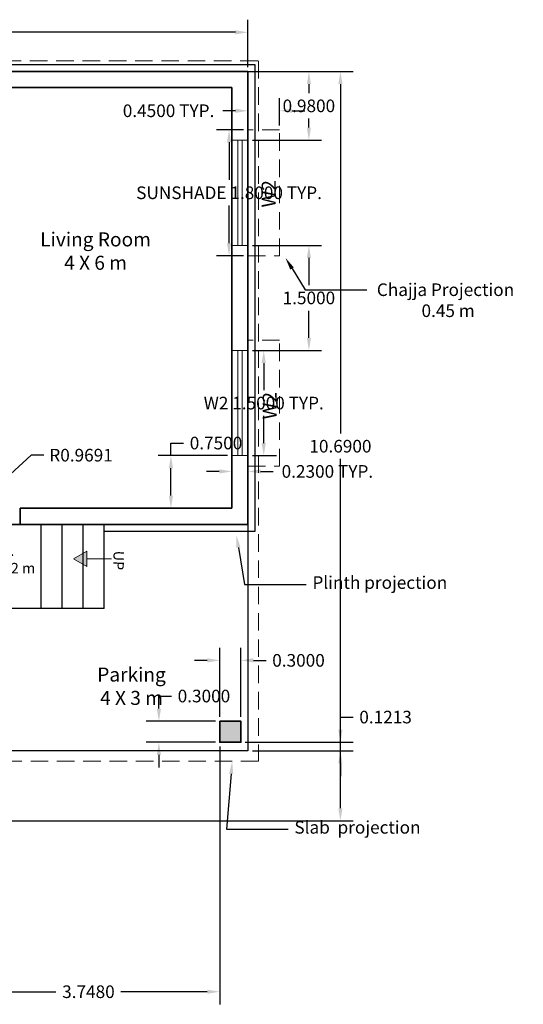
# Model space of a CAD drawing. Units: metres. Extents: x 5.2 to 41.7, y 12.2 to 37.4.
# Tile 4 of 6: x 27.6 to 34.8, y 12.4 to 26.4. Entities that reach past the tile are written whole.
import ezdxf
from ezdxf import colors
from ezdxf.entities.mleader import LeaderData, LeaderLine
from ezdxf.math import Vec2, Vec3

# ---------------------------------------------------------------- set-up
doc = ezdxf.new("R2010")
doc.units = ezdxf.units.M
doc.header["$MEASUREMENT"] = 0
doc.linetypes.add('HIDDEN', pattern=[0.375, 0.25, -0.125])
for name, color, linetype, lineweight in [('A-ANNO-DIMS', 2, 'Continuous', 18), ('A-ANNO-SYMB', 1, 'Continuous', 18), ('A-ANNO-TEXT', 3, 'Continuous', 18), ('A-AREA-IDEN', 3, 'Continuous', 18), ('A-COLS', 1, 'Continuous', 35), ('A-COLS-PATT', 1, 'Continuous', 18), ('A-FLOR-PLIN', 7, 'Continuous', 25), ('A-FLOR-STRS', 7, 'Continuous', 25), ('A-ROOF-OVHD', 252, 'HIDDEN', 18), ('A-WALL', 7, 'Continuous', 35)]:
    doc.layers.add(name, color=color, linetype=linetype, lineweight=lineweight)
doc.layers.add('A-GLAZ', color=51, linetype='Continuous', lineweight=18, true_color=0xf7f281)
doc.styles.get("Standard").update_dxf_attribs({"font": 'arial.ttf'})
doc.dimstyles.get("Standard").update_dxf_attribs({"dimtxt": 0.18, "dimasz": 0.18, "dimexe": 0.18, "dimexo": 0.0625, "dimgap": 0.09, "dimtad": 0, "dimtih": 1, "dimtoh": 1, "dimdec": 4, "dimzin": 0, "dimdsep": 46, "dimtxsty": 'Standard', "dimcen": 0.09, "dimadec": 0, "dimazin": 0, "dimtfac": 1, "dimtdec": 4, "dimtofl": 0, "dimtmove": 0, "dimatfit": 3, "dimfxl": 1, "dimtolj": 1, "dimtzin": 0, "dimarcsym": 0})

# ---------------------------------------------------------------- blocks, each defined once
blk = doc.blocks.new('*D3')
at = {"layer": 'A-ANNO-DIMS', "color": 0, "lineweight": -2, "transparency": 16777216}
for p, q in [((20.753, 25.723), (20.753, 26.4)), ((30.863, 25.723), (30.863, 26.4)), ((20.933, 26.22), (25.283, 26.22)), ((30.683, 26.22), (26.333, 26.22))]:
    blk.add_line(p, q, dxfattribs=at)
at = {"layer": 'A-ANNO-DIMS', "color": 0, "lineweight": 25, "transparency": 16777216}
for points in [[(20.933, 26.25), (20.933, 26.19), (20.753, 26.22)], [(30.683, 26.25), (30.683, 26.19), (30.863, 26.22)]]:
    blk.add_solid(points, dxfattribs=at)
at = {"layer": 'Defpoints', "color": 0, "lineweight": 25, "transparency": 16777216}
for p in [(30.863, 26.22), (20.753, 25.661), (30.863, 25.661)]:
    blk.add_point(p, dxfattribs=at)
at = {"layer": 'A-ANNO-DIMS', "color": 0, "transparency": 16777216, "insert": (25.808, 26.22), "char_height": 0.18, "attachment_point": 5}
blk.add_mtext('\\A1;10.1100', dxfattribs=at)
blk = doc.blocks.new('WIN-W2-1500')
for p, q in [((0.23, 1.5), (0, 1.5)), ((0.085, 1.5), (0.085, 0)), ((0.145, 1.5), (0.145, 0)), ((0.23, 0), (0, 0))]:
    blk.add_line(p, q)
blk = doc.blocks.new('SUNSHADE-W2-1800')
blk.add_lwpolyline([(0.45, 1.65), (0.45, 1.8), (0, 1.8), (0, 0), (0.45, 0), (0.45, 0.15)])
blk = doc.blocks.new('STAIR-DIRECTION')
h = blk.add_hatch(color=256)
h.dxf.hatch_style = 1
h.paths.add_polyline_path([(0.219, 0.189), (0, 0.189), (0.044, 0.113), (0.175, 0.113)])
h.paths.add_polyline_path([(0.175, 0.113), (0.044, 0.113), (0.11, 0)])
blk.add_line((0.11, 0.189), (0.11, 0.542))
blk.add_lwpolyline([(0.11, 0), (0.219, 0.189), (0, 0.189)], close=True)
blk = doc.blocks.new('*D14')
at = {"layer": 'A-ANNO-DIMS', "color": 0, "lineweight": -2, "transparency": 16777216}
for p, q in [((30.926, 21.681), (31.268, 21.681)), ((31.088, 21.501), (31.088, 21.113)), ((31.088, 20.361), (31.088, 20.749)), ((30.926, 20.181), (31.268, 20.181))]:
    blk.add_line(p, q, dxfattribs=at)
at = {"layer": 'A-ANNO-DIMS', "color": 0, "lineweight": 25, "transparency": 16777216}
for points in [[(31.058, 21.501), (31.118, 21.501), (31.088, 21.681)], [(31.058, 20.361), (31.118, 20.361), (31.088, 20.181)]]:
    blk.add_solid(points, dxfattribs=at)
at = {"layer": 'Defpoints', "color": 0, "lineweight": 25, "transparency": 16777216}
for p in [(30.863, 21.681), (31.088, 21.681), (30.863, 20.181)]:
    blk.add_point(p, dxfattribs=at)
at = {"layer": 'A-ANNO-DIMS', "color": 0, "transparency": 16777216, "insert": (31.088, 20.931), "char_height": 0.18, "attachment_point": 5}
blk.add_mtext('\\A1;W2 1.5000 TYP.', dxfattribs=at)
blk = doc.blocks.new('*D15')
at = {"layer": 'A-ANNO-DIMS', "color": 0, "lineweight": -2, "transparency": 16777216}
for p, q in [((30.633, 20.118), (30.633, 19.776)), ((30.863, 20.118), (30.863, 19.776)), ((30.453, 19.956), (30.273, 19.956)), ((31.043, 19.956), (31.223, 19.956))]:
    blk.add_line(p, q, dxfattribs=at)
at = {"layer": 'A-ANNO-DIMS', "color": 0, "lineweight": 25, "transparency": 16777216}
for points in [[(30.453, 19.986), (30.453, 19.926), (30.633, 19.956)], [(31.043, 19.986), (31.043, 19.926), (30.863, 19.956)]]:
    blk.add_solid(points, dxfattribs=at)
at = {"layer": 'Defpoints', "color": 0, "lineweight": 25, "transparency": 16777216}
for p in [(30.633, 20.181), (30.863, 20.181), (30.863, 19.956)]:
    blk.add_point(p, dxfattribs=at)
at = {"layer": 'A-ANNO-DIMS', "color": 0, "transparency": 16777216, "insert": (31.996, 19.956), "char_height": 0.18, "attachment_point": 5}
blk.add_mtext('\\A1;0.2300 TYP.', dxfattribs=at)
blk = doc.blocks.new('*D16')
at = {"layer": 'A-ANNO-DIMS', "color": 0, "lineweight": -2, "transparency": 16777216}
for p, q in [((30.801, 24.831), (30.413, 24.831)), ((30.593, 24.651), (30.593, 24.114)), ((30.593, 23.211), (30.593, 23.748)), ((30.801, 23.031), (30.413, 23.031))]:
    blk.add_line(p, q, dxfattribs=at)
at = {"layer": 'A-ANNO-DIMS', "color": 0, "lineweight": 25, "transparency": 16777216}
for points in [[(30.563, 24.651), (30.623, 24.651), (30.593, 24.831)], [(30.563, 23.211), (30.623, 23.211), (30.593, 23.031)]]:
    blk.add_solid(points, dxfattribs=at)
at = {"layer": 'Defpoints', "color": 0, "lineweight": 25, "transparency": 16777216}
for p in [(30.863, 24.831), (30.593, 23.031), (30.863, 23.031)]:
    blk.add_point(p, dxfattribs=at)
at = {"layer": 'A-ANNO-DIMS', "color": 0, "transparency": 16777216, "insert": (30.593, 23.931), "char_height": 0.18, "attachment_point": 5}
blk.add_mtext('\\A1;SUNSHADE 1.8000 TYP.', dxfattribs=at)
blk = doc.blocks.new('*D17')
at = {"layer": 'A-ANNO-DIMS', "color": 0, "lineweight": -2, "transparency": 16777216}
for p, q in [((30.863, 24.893), (30.863, 25.281)), ((31.313, 24.893), (31.313, 25.281)), ((30.683, 25.101), (30.503, 25.101)), ((31.493, 25.101), (31.673, 25.101))]:
    blk.add_line(p, q, dxfattribs=at)
at = {"layer": 'A-ANNO-DIMS', "color": 0, "lineweight": 25, "transparency": 16777216}
for points in [[(30.683, 25.131), (30.683, 25.071), (30.863, 25.101)], [(31.493, 25.131), (31.493, 25.071), (31.313, 25.101)]]:
    blk.add_solid(points, dxfattribs=at)
at = {"layer": 'Defpoints', "color": 0, "lineweight": 25, "transparency": 16777216}
for p in [(30.863, 25.101), (30.863, 24.831), (31.313, 24.831)]:
    blk.add_point(p, dxfattribs=at)
at = {"layer": 'A-ANNO-DIMS', "color": 0, "transparency": 16777216, "insert": (29.73, 25.101), "char_height": 0.18, "attachment_point": 5}
blk.add_mtext('\\A1;0.4500 TYP.', dxfattribs=at)
blk = doc.blocks.new('*D26')
at = {"layer": 'A-ANNO-DIMS', "color": 0, "lineweight": -2, "transparency": 16777216}
for p, q in [((24.276, 25.661), (32.362, 25.661)), ((32.182, 25.481), (32.182, 20.498)), ((32.182, 15.151), (32.182, 20.134)), ((26.776, 14.971), (32.362, 14.971))]:
    blk.add_line(p, q, dxfattribs=at)
at = {"layer": 'A-ANNO-DIMS', "color": 0, "lineweight": 25, "transparency": 16777216}
for points in [[(32.152, 25.481), (32.212, 25.481), (32.182, 25.661)], [(32.152, 15.151), (32.212, 15.151), (32.182, 14.971)]]:
    blk.add_solid(points, dxfattribs=at)
at = {"layer": 'Defpoints', "color": 0, "lineweight": 25, "transparency": 16777216}
for p in [(24.213, 25.661), (26.713, 14.971), (32.182, 14.971)]:
    blk.add_point(p, dxfattribs=at)
at = {"layer": 'A-ANNO-DIMS', "color": 0, "transparency": 16777216, "insert": (32.182, 20.316), "char_height": 0.18, "attachment_point": 5}
blk.add_mtext('\\A1;10.6900', dxfattribs=at)
blk = doc.blocks.new('*D32')
at = {"layer": 'A-ANNO-DIMS', "color": 0, "lineweight": -2, "transparency": 16777216}
for p, q in [((30.926, 25.661), (31.912, 25.661)), ((31.732, 25.481), (31.732, 25.353)), ((31.732, 24.861), (31.732, 24.989)), ((30.926, 24.681), (31.912, 24.681))]:
    blk.add_line(p, q, dxfattribs=at)
at = {"layer": 'A-ANNO-DIMS', "color": 0, "lineweight": 25, "transparency": 16777216}
for points in [[(31.702, 25.481), (31.762, 25.481), (31.732, 25.661)], [(31.702, 24.861), (31.762, 24.861), (31.732, 24.681)]]:
    blk.add_solid(points, dxfattribs=at)
at = {"layer": 'Defpoints', "color": 0, "lineweight": 25, "transparency": 16777216}
for p in [(30.863, 25.661), (30.863, 24.681), (31.732, 24.681)]:
    blk.add_point(p, dxfattribs=at)
at = {"layer": 'A-ANNO-DIMS', "color": 0, "transparency": 16777216, "insert": (31.732, 25.171), "char_height": 0.18, "attachment_point": 5}
blk.add_mtext('\\A1;0.9800', dxfattribs=at)
blk = doc.blocks.new('*D33')
at = {"layer": 'A-ANNO-DIMS', "color": 0, "lineweight": -2, "transparency": 16777216}
for p, q in [((30.926, 23.181), (31.912, 23.181)), ((31.732, 23.001), (31.732, 22.613)), ((31.732, 21.861), (31.732, 22.249)), ((30.926, 21.681), (31.912, 21.681))]:
    blk.add_line(p, q, dxfattribs=at)
at = {"layer": 'A-ANNO-DIMS', "color": 0, "lineweight": 25, "transparency": 16777216}
for points in [[(31.702, 23.001), (31.762, 23.001), (31.732, 23.181)], [(31.702, 21.861), (31.762, 21.861), (31.732, 21.681)]]:
    blk.add_solid(points, dxfattribs=at)
at = {"layer": 'Defpoints', "color": 0, "lineweight": 25, "transparency": 16777216}
for p in [(30.863, 23.181), (30.863, 21.681), (31.732, 21.681)]:
    blk.add_point(p, dxfattribs=at)
at = {"layer": 'A-ANNO-DIMS', "color": 0, "transparency": 16777216, "insert": (31.732, 22.431), "char_height": 0.18, "attachment_point": 5}
blk.add_mtext('\\A1;1.5000', dxfattribs=at)
blk = doc.blocks.new('*D65')
at = {"layer": 'A-ANNO-DIMS', "color": 0, "lineweight": -2, "transparency": 16777216}
for p, q in [((29.764, 20.181), (29.764, 20.361)), ((29.764, 20.361), (29.944, 20.361)), ((30.571, 20.181), (29.584, 20.181)), ((29.764, 19.611), (29.764, 20.001)), ((30.571, 19.431), (29.584, 19.431))]:
    blk.add_line(p, q, dxfattribs=at)
at = {"layer": 'A-ANNO-DIMS', "color": 0, "lineweight": 25, "transparency": 16777216}
for points in [[(29.734, 20.001), (29.794, 20.001), (29.764, 20.181)], [(29.734, 19.611), (29.794, 19.611), (29.764, 19.431)]]:
    blk.add_solid(points, dxfattribs=at)
at = {"layer": 'Defpoints', "color": 0, "lineweight": 25, "transparency": 16777216}
for p in [(29.764, 20.181), (30.633, 20.181), (30.633, 19.431)]:
    blk.add_point(p, dxfattribs=at)
at = {"layer": 'A-ANNO-DIMS', "color": 0, "transparency": 16777216, "insert": (30.407, 20.361), "char_height": 0.18, "attachment_point": 5}
blk.add_mtext('\\A1;0.7500', dxfattribs=at)
blk = doc.blocks.new('*D66')
at = {"layer": 'A-ANNO-DIMS', "color": 0, "lineweight": -2, "transparency": 16777216}
for p, q in [((30.461, 16.455), (30.461, 17.441)), ((30.761, 16.455), (30.761, 17.441)), ((30.281, 17.261), (30.101, 17.261)), ((30.941, 17.261), (31.121, 17.261))]:
    blk.add_line(p, q, dxfattribs=at)
at = {"layer": 'A-ANNO-DIMS', "color": 0, "lineweight": 25, "transparency": 16777216}
for points in [[(30.281, 17.291), (30.281, 17.231), (30.461, 17.261)], [(30.941, 17.291), (30.941, 17.231), (30.761, 17.261)]]:
    blk.add_solid(points, dxfattribs=at)
at = {"layer": 'Defpoints', "color": 0, "lineweight": 25, "transparency": 16777216}
for p in [(30.761, 17.261), (30.461, 16.392), (30.761, 16.392)]:
    blk.add_point(p, dxfattribs=at)
at = {"layer": 'A-ANNO-DIMS', "color": 0, "transparency": 16777216, "insert": (31.584, 17.261), "char_height": 0.18, "attachment_point": 5}
blk.add_mtext('\\A1;0.3000', dxfattribs=at)
blk = doc.blocks.new('*D67')
at = {"layer": 'A-ANNO-DIMS', "color": 0, "lineweight": -2, "transparency": 16777216}
for p, q in [((29.592, 16.572), (29.592, 16.752)), ((29.592, 16.752), (29.772, 16.752)), ((30.399, 16.392), (29.412, 16.392)), ((30.399, 16.092), (29.412, 16.092)), ((29.592, 15.912), (29.592, 15.732))]:
    blk.add_line(p, q, dxfattribs=at)
at = {"layer": 'A-ANNO-DIMS', "color": 0, "lineweight": 25, "transparency": 16777216}
for points in [[(29.562, 16.572), (29.622, 16.572), (29.592, 16.392)], [(29.562, 15.912), (29.622, 15.912), (29.592, 16.092)]]:
    blk.add_solid(points, dxfattribs=at)
at = {"layer": 'Defpoints', "color": 0, "lineweight": 25, "transparency": 16777216}
for p in [(29.592, 16.392), (30.461, 16.392), (30.461, 16.092)]:
    blk.add_point(p, dxfattribs=at)
at = {"layer": 'A-ANNO-DIMS', "color": 0, "transparency": 16777216, "insert": (30.235, 16.752), "char_height": 0.18, "attachment_point": 5}
blk.add_mtext('\\A1;0.3000', dxfattribs=at)
blk = doc.blocks.new('*D68')
at = {"layer": 'A-ANNO-DIMS', "color": 0, "lineweight": -2, "transparency": 16777216}
for p, q in [((32.182, 16.272), (32.182, 16.452)), ((32.182, 16.452), (32.362, 16.452)), ((30.824, 16.092), (32.362, 16.092)), ((30.926, 15.971), (32.362, 15.971)), ((32.182, 15.791), (32.182, 15.611))]:
    blk.add_line(p, q, dxfattribs=at)
at = {"layer": 'A-ANNO-DIMS', "color": 0, "lineweight": 25, "transparency": 16777216}
for points in [[(32.152, 16.272), (32.212, 16.272), (32.182, 16.092)], [(32.152, 15.791), (32.212, 15.791), (32.182, 15.971)]]:
    blk.add_solid(points, dxfattribs=at)
at = {"layer": 'Defpoints', "color": 0, "lineweight": 25, "transparency": 16777216}
for p in [(30.761, 16.092), (32.182, 16.092), (30.863, 15.971)]:
    blk.add_point(p, dxfattribs=at)
at = {"layer": 'A-ANNO-DIMS', "color": 0, "transparency": 16777216, "insert": (32.826, 16.452), "char_height": 0.18, "attachment_point": 5}
blk.add_mtext('\\A1;0.1213', dxfattribs=at)
blk = doc.blocks.new('*D69')
at = {"layer": 'A-ANNO-DIMS', "color": 0, "lineweight": -2, "transparency": 16777216}
for p, q in [((30.461, 16.03), (30.461, 12.354)), ((26.713, 15.908), (26.713, 12.354)), ((26.893, 12.534), (28.124, 12.534)), ((30.281, 12.534), (29.05, 12.534))]:
    blk.add_line(p, q, dxfattribs=at)
at = {"layer": 'A-ANNO-DIMS', "color": 0, "lineweight": 25, "transparency": 16777216}
for points in [[(26.893, 12.564), (26.893, 12.504), (26.713, 12.534)], [(30.281, 12.564), (30.281, 12.504), (30.461, 12.534)]]:
    blk.add_solid(points, dxfattribs=at)
at = {"layer": 'Defpoints', "color": 0, "lineweight": 25, "transparency": 16777216}
for p in [(30.461, 16.092), (26.713, 15.971), (30.461, 12.534)]:
    blk.add_point(p, dxfattribs=at)
at = {"layer": 'A-ANNO-DIMS', "color": 0, "transparency": 16777216, "insert": (28.587, 12.534), "char_height": 0.18, "attachment_point": 5}
blk.add_mtext('\\A1;3.7480', dxfattribs=at)
blk = doc.blocks.new('*D93')
at = {"layer": 'A-ANNO-DIMS', "color": 0, "lineweight": -2, "transparency": 16777216}
for p, q in [((27.769, 20.188), (27.475, 19.915)), ((27.949, 20.188), (27.769, 20.188)), ((26.543, 19.133), (26.723, 19.133)), ((26.633, 19.043), (26.633, 19.223))]:
    blk.add_line(p, q, dxfattribs=at)
at = {"layer": 'A-ANNO-DIMS', "color": 0, "lineweight": 25, "transparency": 16777216}
blk.add_solid([(27.455, 19.937), (27.496, 19.893), (27.343, 19.792)], dxfattribs=at)
at = {"layer": 'Defpoints', "color": 0, "lineweight": 25, "transparency": 16777216}
for p in [(27.343, 19.792), (26.633, 19.133)]:
    blk.add_point(p, dxfattribs=at)
at = {"layer": 'A-ANNO-DIMS', "color": 0, "transparency": 16777216, "insert": (28.482, 20.188), "char_height": 0.18, "attachment_point": 5}
blk.add_mtext('\\A1;R0.9691', dxfattribs=at)

msp = doc.modelspace()

# ---------------------------------------------------------------- hatches: boundary and pattern name
at = {"layer": 'A-COLS-PATT'}
h = msp.add_hatch(color=256, dxfattribs=at)
h.dxf.hatch_style = 1
h.paths.add_polyline_path([(30.76113, 16.39214), (30.46113, 16.39214), (30.46113, 16.09214), (30.76113, 16.09214)])

# ---------------------------------------------------------------- linework, layer by layer
at = {"layer": 'A-COLS'}
msp.add_lwpolyline([(30.46113, 16.39214), (30.76113, 16.39214), (30.76113, 16.09214), (30.46113, 16.09214)], close=True, dxfattribs=at)
at = {"layer": 'A-FLOR-PLIN'}
for p, q in [((30.86317, 19.20081), (30.86317, 15.97081)), ((30.86317, 15.97081), (26.71317, 15.97081))]:
    msp.add_line(p, q, dxfattribs=at)
msp.add_lwpolyline([(23.90317, 15.87081), (20.65317, 15.87081), (20.65317, 25.76081), (24.31317, 25.76081), (24.31317, 25.18081), (26.30317, 25.18081), (26.30317, 25.76081), (30.96317, 25.76081), (30.96317, 19.10081), (28.81317, 19.10081)], dxfattribs=at)
at = {"layer": 'A-FLOR-STRS'}
for p, q in [((27.91317, 18.00081), (27.91317, 19.20081)), ((28.21317, 18.00081), (28.21317, 19.20081)), ((28.51317, 18.00081), (28.51317, 19.20081)), ((28.81317, 18.00081), (28.81317, 19.20081)), ((28.81317, 18.00081), (26.71317, 18.00081))]:
    msp.add_line(p, q, dxfattribs=at)
at = {"layer": 'A-ROOF-OVHD'}
msp.add_lwpolyline([(23.90317, 15.82081), (20.60317, 15.82081), (20.60317, 25.81081), (24.36317, 25.81081), (24.36317, 25.23081), (26.25317, 25.23081), (26.25317, 25.81081), (31.01317, 25.81081), (31.01317, 15.82081), (26.71317, 15.82081)], dxfattribs=at)
at = {"layer": 'A-WALL'}
for p, q in [((30.86317, 25.66081), (26.40317, 25.66081)), ((30.86317, 19.20081), (30.86317, 25.66081)), ((30.63317, 25.43081), (26.63317, 25.43081)), ((30.63317, 22.43081), (30.63317, 25.43081)), ((30.63317, 19.43081), (30.63317, 22.43081)), ((30.63317, 19.43081), (27.61317, 19.43081)), ((27.61317, 19.20081), (27.61317, 19.43081)), ((30.86317, 19.20081), (26.71317, 19.20081))]:
    msp.add_line(p, q, dxfattribs=at)

# ---------------------------------------------------------------- block references
at = {"layer": 'A-ANNO-SYMB', "rotation": 269.9999999999995}
msp.add_blockref('STAIR-DIRECTION', (28.37556, 18.82005), dxfattribs=at)
at = {"layer": 'A-GLAZ'}
for p in [(30.633, 23.181), (30.633, 20.181)]:
    msp.add_blockref('WIN-W2-1500', p, dxfattribs=at)
at = {"layer": 'A-ROOF-OVHD', "rotation": 180}
for p in [(31.31334, 24.83062), (31.31334, 21.83062)]:
    msp.add_blockref('SUNSHADE-W2-1800', p, dxfattribs=at)

# ---------------------------------------------------------------- texts
at = {"layer": 'A-ANNO-TEXT', "attachment_point": 1}
for s, insert, char_height, rotation in [('\\pxqc;{W2 }', (31.0589, 22.99244), 0.2, 90), ('\\pxqc;{W2 }', (31.07241, 19.96981), 0.2, 90), ('\\pxqc;{UP }', (29.11081, 19.60871), 0.15, 268.903059)]:
    msp.add_mtext_dynamic_manual_height_columns(s, width=1.8483261, gutter_width=1, heights=[0], dxfattribs=dict(at, insert=insert, char_height=char_height, rotation=rotation))
at = {"layer": 'A-AREA-IDEN', "attachment_point": 1}
for s, insert, char_height in [('\\pxqc;{Living Room \\P4 X 6 m }', (27.76446, 23.36586), 0.2), ('\\pxqc;{Ver .\\P1.2 X 1.2 m}', (26.39866, 18.90081), 0.15), ('\\pxqc;{Parking  \\P4 X 3 m}', (28.2775, 17.15862), 0.2)]:
    msp.add_mtext_dynamic_manual_height_columns(s, width=1.8483261, gutter_width=1, heights=[0], dxfattribs=dict(at, insert=insert, char_height=char_height))

# ---------------------------------------------------------------- dimensions: what is measured, and where the dimension line sits
at = {"layer": 'A-ANNO-DIMS'}
for base, p1, p2, override, picture, middle in [((30.86317, 26.22005), (20.75317, 25.66081), (30.86317, 25.66081), {"dimclrd": 0, "dimclre": 0, "dimclrt": 0}, '*D3', (25.80817, 26.22005)), ((30.76113, 17.26114), (30.46113, 16.39214), (30.76113, 16.39214), {"dimdec": 4, "dimlfac": 1, "dimrnd": 0, "dimzin": 0, "dimdsep": 46, "dimlunit": 2}, '*D66', (31.58445, 17.26114)), ((30.46113, 12.53449), (26.71317, 15.97081), (30.46113, 16.09214), {"dimdec": 4, "dimlfac": 1, "dimrnd": 0, "dimzin": 0, "dimdsep": 46, "dimlunit": 2}, '*D69', (28.58715, 12.53449))]:
    dim = msp.add_linear_dim(base=base, p1=p1, p2=p2, dimstyle='Standard', override=override, dxfattribs=at)
    dim.commit()
    dim.dimension.update_dxf_attribs({"geometry": picture, "text_midpoint": middle})
for base, p1, p2, angle, picture, middle in [((32.18217, 14.97081), (24.21317, 25.66081), (26.71317, 14.97081), 90, '*D26', (32.18217, 20.31581)), ((31.73217, 24.68081), (30.86317, 25.66081), (30.86317, 24.68081), 270, '*D32', (31.73217, 25.17081)), ((31.73217, 21.68081), (30.86317, 23.18081), (30.86317, 21.68081), 270, '*D33', (31.73217, 22.43081)), ((29.76417, 20.18081), (30.63317, 19.43081), (30.63317, 20.18081), 90, '*D65', (30.40749, 20.36081)), ((29.59213, 16.39214), (30.46113, 16.09214), (30.46113, 16.39214), 90, '*D67', (30.23545, 16.75214)), ((32.18217, 16.09214), (30.86317, 15.97081), (30.76113, 16.09214), 90, '*D68', (32.8258, 16.45214))]:
    dim = msp.add_linear_dim(base=base, p1=p1, p2=p2, angle=angle, dimstyle='Standard', override={"dimdec": 4, "dimlfac": 1, "dimrnd": 0, "dimzin": 0, "dimdsep": 46, "dimlunit": 2}, dxfattribs=at)
    dim.commit()
    dim.dimension.update_dxf_attribs({"geometry": picture, "text_midpoint": middle})
for base, p1, p2, angle, text, picture, middle in [((30.86317, 25.10081), (31.31317, 24.83081), (30.86317, 24.83081), 180, '<> TYP.', '*D17', (29.73037, 25.10081)), ((30.59317, 23.03081), (30.86317, 24.83081), (30.86317, 23.03081), 270, 'SUNSHADE <> TYP.', '*D16', (30.59317, 23.93081)), ((31.08817, 21.68081), (30.86317, 20.18081), (30.86317, 21.68081), 90, 'W2 <> TYP.', '*D14', (31.08817, 20.93081))]:
    dim = msp.add_linear_dim(base=base, p1=p1, p2=p2, angle=angle, text=text, dimstyle='Standard', override={"dimdec": 4, "dimlfac": 1, "dimrnd": 0, "dimzin": 0, "dimdsep": 46, "dimlunit": 2}, dxfattribs=at)
    dim.commit()
    dim.dimension.update_dxf_attribs({"geometry": picture, "text_midpoint": middle})
dim = msp.add_radius_dim(center=(26.632909, 19.132957), mpoint=(27.343186, 19.792173), dimstyle='Standard', override={"dimdec": 4, "dimlfac": 1, "dimrnd": 0, "dimzin": 0, "dimdsep": 46, "dimlunit": 2}, dxfattribs=at)
dim.commit()
dim.dimension.update_dxf_attribs({"geometry": '*D93', "text_midpoint": (28.481739, 20.187702), "dimtype": 164})
dim = msp.add_linear_dim(base=(30.86317, 19.95581), p1=(30.63317, 20.18081), p2=(30.86317, 20.18081), text='<> TYP.', dimstyle='Standard', override={"dimdec": 4, "dimlfac": 1, "dimrnd": 0, "dimzin": 0, "dimdsep": 46, "dimlunit": 2}, dxfattribs=at)
dim.commit()
dim.dimension.update_dxf_attribs({"geometry": '*D15', "text_midpoint": (31.99597, 19.95581)})

# ---------------------------------------------------------------- leaders
at = {"layer": 'A-ANNO-TEXT'}
ml = msp.add_multileader_mtext('Standard', dxfattribs=at)
ml.set_content(' Chajja Projection\\P\\pxqc;0.45 m  ', color=256)
ml.set_leader_properties()
ml.build(insert=Vec2(0, 0))
ml.multileader.update_dxf_attribs({"dogleg_length": 0.36, "arrow_head_size": 0.18})
ctx = ml.context
ctx.base_point, ctx.char_height, ctx.arrow_head_size, ctx.landing_gap_size, ctx.plane_origin = Vec3(32.55623, 22.54682), 0.18, 0.18, 0.09, Vec3(31.32565, 22.89848)
notes = []
notes.append((ctx, [(0, (1, 1, 0), (31.67926, 22.54682), (1, 0), 0.87697, [(0, [(31.39707, 23.00368)], 0, [])])]))
ctx.mtext.insert, ctx.mtext.width, ctx.mtext.flow_direction = Vec3(32.64623, 22.63836), 2.1445866, 5
ml = msp.add_multileader_mtext('Standard', dxfattribs=at)
ml.set_content('Plinth projection ', color=256)
ml.set_leader_properties()
ml.build(insert=Vec2(0, 0))
ml.multileader.update_dxf_attribs({"dogleg_length": 0.36, "arrow_head_size": 0.18})
ctx = ml.context
ctx.base_point, ctx.char_height, ctx.arrow_head_size, ctx.landing_gap_size, ctx.plane_origin = Vec3(31.69247, 18.3443), 0.18, 0.18, 0.09, Vec3(30.62556, 18.94244)
notes.append((ctx, [(0, (1, 1, 0), (30.8155, 18.3443), (1, 0), 0.87697, [(0, [(30.69698, 19.04764)], 0, [])])]))
ctx.mtext.insert, ctx.mtext.flow_direction = Vec3(31.78247, 18.46076), 5
ml = msp.add_multileader_mtext('Standard', dxfattribs=at)
ml.set_content('Slab  projection ', color=256)
ml.set_leader_properties()
ml.build(insert=Vec2(0, 0))
ml.multileader.update_dxf_attribs({"dogleg_length": 0.36, "arrow_head_size": 0.18})
ctx = ml.context
ctx.base_point, ctx.char_height, ctx.arrow_head_size, ctx.landing_gap_size, ctx.plane_origin = Vec3(31.43479, 14.85251), 0.18, 0.18, 0.09, Vec3(30.4277, 15.63365)
notes.append((ctx, [(0, (1, 1, 0), (30.55782, 14.85251), (1, 0), 0.87697, [(0, [(30.63787, 15.82081)], 0, [])])]))
ctx.mtext.insert, ctx.mtext.flow_direction = Vec3(31.52479, 14.96897), 5
for ctx, leaders in notes:
    for number, flags, end, landing, length, lines in leaders:
        leader = LeaderData()
        leader.index, (leader.has_last_leader_line, leader.has_dogleg_vector, leader.attachment_direction) = number, flags
        leader.last_leader_point, leader.dogleg_vector, leader.dogleg_length = Vec3(end), Vec3(landing), length
        for number, points, colour, breaks in lines:
            line = LeaderLine()
            line.index, line.vertices, line.color, line.breaks = number, Vec3.list(points), colors.encode_raw_color(colour), breaks
            leader.lines.append(line)
        ctx.leaders.append(leader)

doc.saveas('drawing.dxf')
